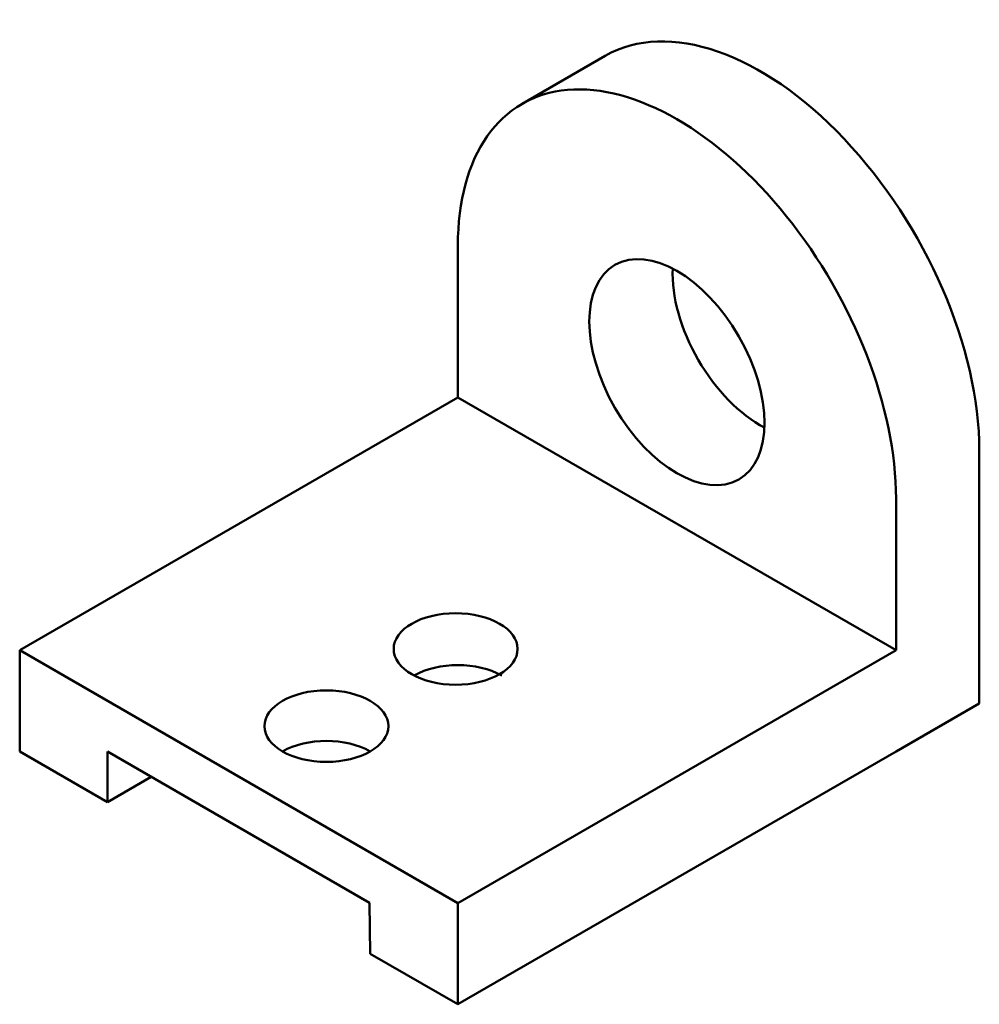
# Model space of a CAD drawing. Units: millimetres. Extents: x 567 to 661.8, y -242.3 to -144.9.
import ezdxf

# ---------------------------------------------------------------- set-up
doc = ezdxf.new("R2010")
doc.units = ezdxf.units.MM
doc.header["$MEASUREMENT"] = 0
doc.layers.add('M-OUTL', color=7, linetype='Continuous', lineweight=50)

msp = doc.modelspace()

# ---------------------------------------------------------------- linework, layer by layer
at = {"layer": 'M-OUTL'}
for p, q in [((624.851, -148.494), (616.624, -153.244)), ((610.283, -182.261), (610.283, -167.261)), ((566.981, -207.261), (610.283, -182.261)), ((653.584, -207.261), (610.283, -182.261)), ((661.809, -201.574), (661.809, -186.574)), ((653.584, -207.261), (653.584, -192.261)), ((661.809, -201.574), (661.809, -212.512)), ((566.981, -207.261), (610.283, -232.261)), ((566.981, -207.261), (566.981, -217.261)), ((610.283, -232.261), (653.584, -207.261)), ((653.584, -217.261), (661.809, -212.512)), ((575.642, -222.261), (566.981, -217.261)), ((575.642, -222.261), (575.642, -217.261)), ((575.642, -217.261), (601.547, -232.218)), ((610.283, -242.261), (653.584, -217.261)), ((579.972, -219.761), (575.642, -222.261)), ((579.972, -219.761), (580.07, -219.704)), ((601.622, -237.261), (601.547, -232.218)), ((610.283, -232.261), (610.283, -242.261)), ((610.283, -242.261), (601.622, -237.261))]:
    msp.add_line(p, q, dxfattribs=at)
for centre, major_axis, start_param, end_param in [((640.161, -175.011), (15.309, -26.517), 0.785398, 3.141593), ((631.933, -179.761), (15.309, -26.517), 0.785398, 3.926991), ((640.161, -175.011), (6.124, -10.607), 3.878163, 5.546615), ((610.283, -212.261), (6.124, 0), 0.785398, 2.356194), ((597.293, -219.761), (6.124, 0), 0.785398, 2.356194)]:
    msp.add_ellipse(centre, major_axis=major_axis, ratio=0.57735, start_param=start_param, end_param=end_param, dxfattribs=at)
for centre, major_axis in [((631.933, -179.761), (6.124, -10.607)), ((610.062, -207.133), (-6.124, 0)), ((597.292, -214.761), (-6.124, 0))]:
    msp.add_ellipse(centre, major_axis=major_axis, ratio=0.57735, dxfattribs=at)

doc.saveas('drawing.dxf')
